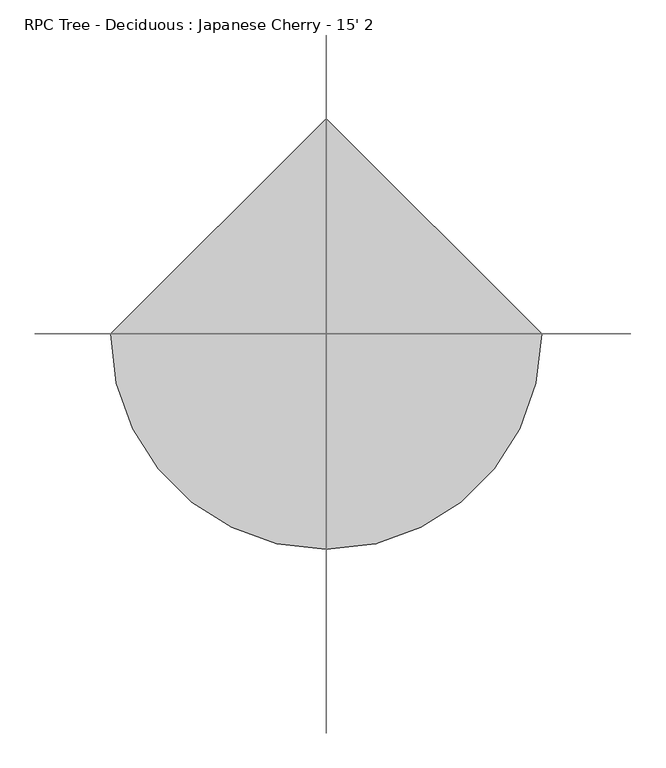
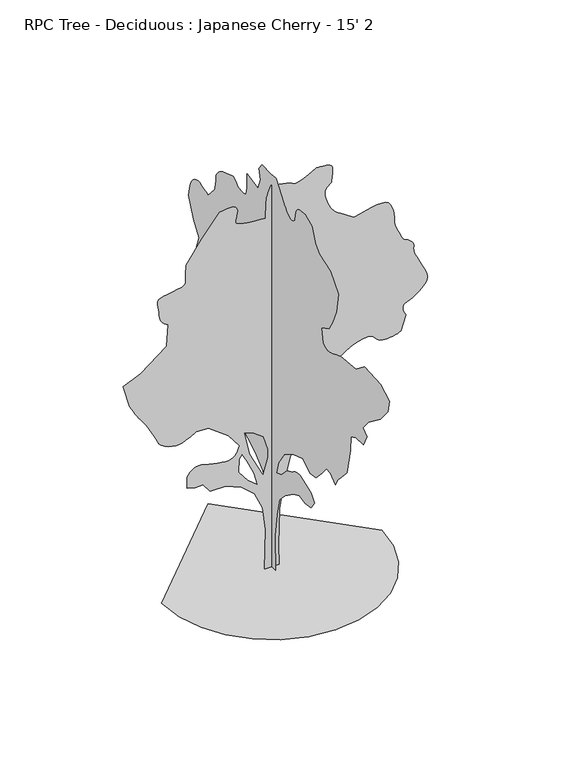
"""IFC4 building model written with IfcOpenShell, lengths in millimetres: geographic element geometry, RPC Tree - Deciduous : Japanese Cherry - 15' 2."""

from ifc_helpers import new_model, si_unit, origin, place, context, project, spatial, triangles, source, transform, mapped, element, save


def rpc_tree_deciduous_japanese_cherry_15_2_e499737d(model_context):
    return source(origin(), model_context, "Body", "Tessellation", [
        triangles([(-0.0028028, 75.7657196, 0.0059537), (-0.0028028, -73.2478183, 0.0059537), (-0.0028028, -59.7012251, 399.6312029), (-0.0028028, -100.3410047, 663.7914597), (-0.0028028, -147.7544623, 866.9916292), (-0.0028028, -256.1287339, 982.1375078), (-0.0028028, -418.6863261, 1097.2859299), (-0.0028028, -527.0605977, 1144.6976435), (-0.0028028, -635.434833, 1124.3775902), (-0.0028028, -750.5807842, 1144.6976435), (-0.0028028, -811.5407988, 1232.7519344), (-0.0028028, -750.5807842, 1314.0320023), (-0.0028028, -533.8347845, 1388.5377743), (-0.0028028, -514.9955638, 1387.0189716), (-0.0028028, -496.3341665, 1385.0834793), (-0.0028028, -478.0283798, 1382.3173691), (-0.0028028, -460.2559908, 1378.3091835), (-0.0028028, -443.1947865, 1372.6425236), (-0.0028028, -427.0200471, 1364.9005543), (-0.0028028, -411.9146828, 1354.6719635), (-0.0028028, -396.8067387, 1343.65345), (-0.0028028, -380.6345427, 1333.6991158), (-0.0028028, -363.5733384, 1324.6364422), (-0.0028028, -345.8009494, 1316.2824463), (-0.0028028, -327.4951627, 1308.4643188), (-0.0028028, -308.8337654, 1300.9992222), (-0.0028028, -289.994581, 1293.7118763), (-0.0028028, -188.3942419, 1185.3376774), (-0.0028028, -86.7944115, 1144.6976435), (-0.0028028, -127.4344454, 1286.9377258), (-0.0028028, -242.580869, 1456.2720119), (-0.0028028, -405.140496, 1557.8722057), (-0.0028028, -594.794799, 1618.8321476), (-0.0028028, -730.2607309, 1530.7779293), (-0.0028028, -838.6350025, 1544.3263756), (-0.0028028, -953.7809538, 1666.2439339), (-0.0028028, -1041.8351721, 1774.6181328), (-0.0028028, -1123.1126965, 1767.8439823), (-0.0028028, -1211.1669147, 1686.5663853), (-0.0028028, -1265.3528515, 1781.3922832), (-0.0028028, -1326.3127934, 1849.1240501), (-0.0028028, -1434.6871376, 1964.2723995), (-0.0028028, -1502.4187592, 2269.0726902), (-0.0028028, -1509.193055, 2431.6328259), (-0.0028028, -1604.0214237, 2472.2703163), (-0.0028028, -1753.0332584, 2485.8186172), (-0.0028028, -1813.9932003, 2614.5002975), (-0.0028028, -1739.4874283, 2675.4602394), (-0.0028028, -1841.0874767, 2797.3804138), (-0.0028028, -2071.3792339, 2973.5042564), (-0.0028028, -2220.3935394, 3149.6025192), (-0.0028028, -2247.4851997, 3291.8426743), (-0.0028028, -2078.1535297, 3386.6610146), (-0.0028028, -1766.5790886, 3400.2244308), (-0.0028028, -1610.7931034, 3278.3045471), (-0.0028028, -1312.7669632, 3244.4208595), (-0.0028028, -1272.2845505, 3228.5456657), (-0.0028028, -1232.7519344, 3213.2041603), (-0.0028028, -1195.1115721, 3198.9294502), (-0.0028028, -1160.3186377, 3186.2546425), (-0.0028028, -1129.3153702, 3175.7137161), (-0.0028028, -1103.0517843, 3167.8397781), (-0.0028028, -1082.4726625, 3163.1406464), (-0.0028028, -1064.0500225, 3162.8865921), (-0.0028028, -1044.5580437, 3166.9000099), (-0.0028028, -1025.4242552, 3173.6309944), (-0.0028028, -1008.065867, 3181.5558014), (-0.0028028, -993.907865, 3189.1248161), (-0.0028028, -984.3701477, 3194.789296), (-0.0028028, -980.8726141, 3197.024334), (-0.0028028, -947.0067307, 3359.5844696), (-0.0028028, -1089.2468857, 3434.0828293), (-0.0028028, -1156.9810507, 3542.4645859), (-0.0028028, -1231.4868954, 3718.5628487), (-0.0028028, -1272.127002, 3942.0832169), (-0.0028028, -1116.3410168, 4118.1814796), (-0.0028028, -913.1409199, 4192.7051285), (-0.0028028, -831.8608521, 4267.2034882), (-0.0028028, -770.9007648, 4429.7636238), (-0.0028028, -628.6606825, 4483.9417122), (-0.0028028, -605.4958537, 4483.8402649), (-0.0028028, -582.6891789, 4483.1542603), (-0.0028028, -560.5911455, 4481.2747238), (-0.0028028, -539.5599438, 4477.6426781), (-0.0028028, -519.9511116, 4471.5974075), (-0.0028028, -502.1202959, 4462.6310944), (-0.0028028, -486.4205638, 4450.0836044), (-0.0028028, -473.6824242, 4434.3863068), (-0.0028028, -464.1447433, 4416.5554184), (-0.0028028, -457.2740144, 4396.9467316), (-0.0028028, -452.5343691, 4375.9154572), (-0.0028028, -449.3949532, 4353.8173874), (-0.0028028, -447.3197528, 4331.0083145), (-0.0028028, -445.7805299, 4307.8434494), (-0.0028028, -434.0914178, 4294.9401672), (-0.0028028, -421.9248276, 4283.0531021), (-0.0028028, -408.8133096, 4273.1978897), (-0.0028028, -394.279422, 4266.3398781), (-0.0028028, -377.850701, 4263.5202827), (-0.0028028, -359.0495956, 4265.7303223), (-0.0028028, -337.4062583, 4273.9853416), (-0.0028028, -315.9610193, 4285.9741447), (-0.0028028, -297.7161846, 4298.6995308), (-0.0028028, -282.1358129, 4312.0091835), (-0.0028028, -268.6864885, 4325.8013649), (-0.0028028, -256.8373934, 4339.9237587), (-0.0028028, -246.0563473, 4354.3002068), (-0.0028028, -235.8074452, 4368.8033913), (-0.0028028, -140.9810386, 4497.5054192), (-0.0028028, -80.0209877, 4572.0037788), (-0.0028028, 21.579147, 4565.2219254), (-0.0028028, 184.1389784, 4572.0037788), (-0.0028028, 245.0987749, 4490.7235657), (-0.0028028, 218.0055885, 4375.5852448), (-0.0028028, 265.4200454, 4246.8835075), (-0.0028028, 475.3918765, 4287.5234688), (-0.0028028, 475.3918765, 4138.5014603), (-0.0028028, 476.9514107, 4115.4383331), (-0.0028028, 479.1637756, 4093.1623672), (-0.0028028, 482.6791134, 4072.5630432), (-0.0028028, 488.1502911, 4054.4781006), (-0.0028028, 496.2249435, 4039.6699928), (-0.0028028, 507.5609885, 4029.0273285), (-0.0028028, 522.8060609, 4023.3631393), (-0.0028028, 540.2228757, 4021.2551285), (-0.0028028, 557.6396542, 4020.5691238), (-0.0028028, 575.056469, 4021.0519432), (-0.0028028, 592.4732474, 4022.4995293), (-0.0028028, 609.8900259, 4024.6586998), (-0.0028028, 627.3093842, 4027.2748192), (-0.0028028, 644.726199, 4030.1449928), (-0.0028028, 660.7002239, 4045.9437378), (-0.0028028, 676.7352917, 4060.8791634), (-0.0028028, 692.8896835, 4074.0362091), (-0.0028028, 709.2193554, 4084.5265572), (-0.0028028, 725.7878208, 4091.4607269), (-0.0028028, 742.6534338, 4093.9498192), (-0.0028028, 759.8720776, 4091.1049347), (-0.0028028, 942.7522665, 4030.1449928), (-0.0028028, 968.7009007, 4012.6698967), (-0.0028028, 993.5827394, 3994.8390083), (-0.0028028, 1016.3309875, 3976.2971169), (-0.0028028, 1035.8813931, 3956.6881393), (-0.0028028, 1051.1646172, 3935.6568649), (-0.0028028, 1061.1163353, 3912.8477921), (-0.0028028, 1064.6722956, 3887.9048378), (-0.0028028, 1065.462291, 3862.3526184), (-0.0028028, 1067.6745832, 3837.8921928), (-0.0028028, 1071.0705969, 3814.3209572), (-0.0028028, 1075.4140091, 3791.4610153), (-0.0028028, 1080.4685698, 3769.1088913), (-0.0028028, 1085.9981741, 3747.1381393), (-0.0028028, 1091.7640285, 3725.3447021), (-0.0028028, 1220.4582081, 3583.1045471), (-0.0028028, 1259.5970982, 3600.2497215), (-0.0028028, 1298.4413841, 3615.8705704), (-0.0028028, 1336.691375, 3628.418351), (-0.0028028, 1374.0521759, 3636.343158), (-0.0028028, 1410.2294735, 3638.0956673), (-0.0028028, 1444.9259022, 3632.1521347), (-0.0028028, 1477.8442417, 3616.9629456), (-0.0028028, 1506.4193871, 3593.4931572), (-0.0028028, 1528.9517326, 3564.3086014), (-0.0028028, 1546.4471764, 3530.3996246), (-0.0028028, 1559.9143776, 3492.7059952), (-0.0028028, 1570.361269, 3452.1674812), (-0.0028028, 1578.7941845, 3409.7241417), (-0.0028028, 1586.218586, 3366.3410339), (-0.0028028, 1498.1643677, 3136.0643921), (-0.0028028, 1389.7926395, 2987.0423836), (-0.0028028, 1477.8442417, 2743.2023254), (-0.0028028, 1396.5641739, 2614.5002975), (-0.0028028, 1363.3893093, 2602.8164177), (-0.0028028, 1331.4588455, 2590.6497185), (-0.0028028, 1302.0151485, 2577.543251), (-0.0028028, 1276.3027645, 2563.0144867), (-0.0028028, 1255.5687103, 2546.5806061), (-0.0028028, 1241.0552067, 2527.7820442), (-0.0028028, 1234.0040382, 2506.1385979), (-0.0028028, 1231.6953129, 2483.1135498), (-0.0028028, 1230.4506214, 2460.4416779), (-0.0028028, 1230.0949745, 2438.0692062), (-0.0028028, 1230.4506214, 2415.9330574), (-0.0028028, 1231.339666, 2393.9721886), (-0.0028028, 1232.5842121, 2372.13326), (-0.0028028, 1234.0040382, 2350.3502872), (-0.0028028, 1206.9124506, 2241.9785591), (-0.0028028, 1017.2581112, 2262.2985397), (-0.0028028, 1001.4999161, 2230.5052769), (-0.0028028, 986.9863398, 2199.5401611), (-0.0028028, 974.9594576, 2170.2361359), (-0.0028028, 966.6663591, 2143.4188774), (-0.0028028, 963.3491198, 2119.9211838), (-0.0028028, 966.2523582, 2100.5664059), (-0.0028028, 976.6180773, 2086.1925739), (-0.0028028, 993.4227201, 2074.2646683), (-0.0028028, 1014.0196461, 2062.1005852), (-0.0028028, 1037.2225176, 2050.292149), (-0.0028028, 1061.8478313, 2039.431184), (-0.0028028, 1086.7093952, 2030.1093693), (-0.0028028, 1110.6234879, 2022.9211452), (-0.0028028, 1132.4039898, 2018.4583363), (-0.0028028, 1152.1322187, 2014.567004), (-0.0028028, 1170.7936523, 2008.9003441), (-0.0028028, 1188.5660414, 2001.7526699), (-0.0028028, 1205.6272093, 1993.4190216), (-0.0028028, 1222.157523, 1984.1961834), (-0.0028028, 1238.3297916, 1974.3816662), (-0.0028028, 1254.3241642, 1964.2723995), (-0.0028028, 1410.1126202, 2045.5524673), (-0.0028028, 1454.8979679, 2056.9850544), (-0.0028028, 1498.4412403, 2067.3533169), (-0.0028028, 1539.4952751, 2075.5879887), (-0.0028028, 1576.817997, 2080.6222744), (-0.0028028, 1609.1650051, 2081.3919949), (-0.0028028, 1635.2914627, 2076.8326801), (-0.0028028, 1653.9502075, 2065.8725933), (-0.0028028, 1666.2946575, 2049.9747265), (-0.0028028, 1674.7249569, 2031.5900928), (-0.0028028, 1679.8989143, 2011.1329113), (-0.0028028, 1682.4669262, 1989.0146393), (-0.0028028, 1683.0789528, 1965.6542919), (-0.0028028, 1682.3881519, 1941.4631813), (-0.0028028, 1681.0444839, 1916.8582878), (-0.0028028, 1657.7627655, 1892.3904499), (-0.0028028, 1634.1255455, 1869.1697742), (-0.0028028, 1609.7770317, 1848.4331039), (-0.0028028, 1584.3618679, 1831.4303627), (-0.0028028, 1557.5241165, 1819.4059513), (-0.0028028, 1528.9110374, 1813.5996197), (-0.0028028, 1498.1643677, 1815.2582394), (-0.0028028, 1465.6015297, 1822.4057682), (-0.0028028, 1432.5637207, 1830.9782101), (-0.0028028, 1400.2370602, 1839.0732101), (-0.0028028, 1369.8078129, 1844.8009129), (-0.0028028, 1342.4571568, 1846.2614342), (-0.0028028, 1319.3735367, 1841.5624477), (-0.0028028, 1301.7382759, 1828.8040695), (-0.0028028, 1288.4084209, 1812.3752758), (-0.0028028, 1277.2120113, 1797.7219551), (-0.0028028, 1267.7912201, 1784.5521194), (-0.0028028, 1259.7953419, 1772.5657871), (-0.0028028, 1252.8636429, 1761.4660286), (-0.0028028, 1246.6430923, 1750.9605652), (-0.0028028, 1240.778334, 1740.752322), (-0.0028028, 1263.8618088, 1737.6916077), (-0.0028028, 1286.1172817, 1733.6834221), (-0.0028028, 1306.714135, 1727.7779686), (-0.0028028, 1324.821896, 1719.0302467), (-0.0028028, 1339.6122723, 1706.4901691), (-0.0028028, 1350.2574074, 1689.2105553), (-0.0028028, 1355.9242126, 1666.2439339), (-0.0028028, 1358.2355541, 1639.3300243), (-0.0028028, 1359.4802456, 1610.9912018), (-0.0028028, 1359.8357471, 1581.4687305), (-0.0028028, 1359.4802456, 1550.9989334), (-0.0028028, 1358.591201, 1519.8178425), (-0.0028028, 1357.3466549, 1488.1643967), (-0.0028028, 1355.9242126, 1456.2720119), (-0.0028028, 1321.1312782, 1430.3436527), (-0.0028028, 1286.5720505, 1405.5990875), (-0.0028028, 1252.4876484, 1383.2266159), (-0.0028028, 1219.1146128, 1364.4078518), (-0.0028028, 1186.6915192, 1350.328624), (-0.0028028, 1155.4494581, 1342.1725811), (-0.0028028, 1125.6323828, 1341.1261333), (-0.0028028, 1095.812764, 1344.8167511), (-0.0028028, 1064.5732464, 1349.9322819), (-0.0028028, 1032.1476093, 1356.2316067), (-0.0028028, 998.774501, 1363.478112), (-0.0028028, 964.6902443, 1371.4385273), (-0.0028028, 930.1334873, 1379.8688267), (-0.0028028, 895.3380095, 1388.5377743), (-0.0028028, 692.1378399, 1341.1261333), (-0.0028028, 455.0718596, 1219.2061043), (-0.0028028, 319.6059277, 1144.6976435), (-0.0028028, 163.8189614, 1016.005862), (-0.0028028, 68.9922959, 819.5799156), (-0.0028028, 41.8991095, 541.8713216), (-0.0028028, 68.9922959, 264.1652892), (80.2102203, 0.0002552, 0.0), (-82.349661, 0.0002552, 0.0), (-68.8030678, 0.0002233, 460.5862032), (-102.6694236, 0.000202, 724.7463873), (-190.7229152, 0.0001914, 914.3981833), (-332.9637969, 0.0001914, 1043.0925081), (-509.0697627, 0.0001807, 1117.5983528), (-678.4015417, 0.0001807, 1117.5983528), (-759.684153, 0.0001807, 1219.1984013), (-847.7358278, 0.0001807, 1219.1984013), (-935.7901188, 0.0001807, 1239.5183819), (-935.7901188, 0.0001701, 1368.2127068), (-918.2539072, 0.0001701, 1391.2175526), (-900.0065472, 0.0001701, 1412.9192802), (-880.3392883, 0.0001595, 1432.0150623), (-858.5384388, 0.0001595, 1447.2017807), (-833.8928501, 0.0001595, 1457.1737011), (-805.6936993, 0.0001595, 1460.6307575), (-773.2299831, 0.0001595, 1456.266925), (-734.6829174, 0.0001595, 1446.5108345), (-690.4487715, 0.0001595, 1435.4516258), (-643.1335636, 0.0001701, 1424.2757092), (-595.3460009, 0.0001701, 1414.1639717), (-549.689449, 0.0001701, 1406.3051491), (-508.7725788, 0.0001701, 1401.8804192), (-475.2013721, 0.0001701, 1402.0785175), (-448.544024, 0.0001701, 1408.1415195), (-426.1513865, 0.0001701, 1419.8916744), (-407.3122021, 0.0001595, 1436.3813656), (-391.3152497, 0.0001595, 1456.660651), (-377.4544679, 0.0001595, 1479.7848209), (-365.0135485, 0.0001595, 1504.8039333), (-353.2838139, 0.0001595, 1530.7728424), (-475.2013721, 0.0001488, 1693.3329781), (-698.7215223, 0.0001382, 1855.8931137), (-834.1899977, 0.0001382, 1862.6647934), (-856.0492739, 0.0001382, 1849.6320133), (-878.4419477, 0.0001382, 1836.7771294), (-901.9038877, 0.0001382, 1824.277747), (-926.9610065, 0.0001382, 1812.3092915), (-954.1543322, 0.0001382, 1801.0544552), (-984.01203, 0.0001382, 1790.6861927), (-1017.0701866, 0.0001488, 1781.3847256), (-1055.1015862, 0.0001488, 1778.1664627), (-1097.4002398, 0.0001488, 1784.6638859), (-1140.7656887, 0.0001382, 1798.9792912), (-1182.0000904, 0.0001382, 1819.2206429), (-1217.9005154, 0.0001382, 1843.490237), (-1245.2690483, 0.0001382, 1869.8935673), (-1260.907774, 0.0001382, 1896.5332203), (-1274.5551968, 0.0001382, 1929.7461639), (-1296.2570698, 0.0001276, 1973.9803825), (-1323.2903034, 0.0001276, 2024.4959038), (-1352.9320988, 0.0001276, 2076.5482498), (-1382.45457, 0.0001276, 2125.4025352), (-1409.1321568, 0.0001169, 2166.3195145), (-1430.2420601, 0.0001169, 2194.5592152), (-1448.055217, 0.0001169, 2217.0508656), (-1466.5769062, 0.0001169, 2243.4541958), (-1485.6928905, 0.0001169, 2273.113868), (-1505.2813751, 0.0001169, 2305.3794857), (-1525.2255066, 0.0001063, 2339.6035595), (-1545.4082863, 0.0001063, 2375.12799), (-1565.7080647, 0.0001063, 2411.3051422), (-1640.2164528, 9.57e-05, 2668.7039658), (-1443.7878902, 8.51e-05, 2749.9838882), (-1159.310269, 7.44e-05, 2973.5042564), (-1145.7618954, 5.32e-05, 3217.3190254), (-1165.9447477, 5.32e-05, 3231.9748169), (-1185.2970549, 5.32e-05, 3247.3163223), (-1202.9906696, 5.32e-05, 3264.0804153), (-1218.1951195, 5.32e-05, 3282.9780991), (-1230.0823299, 5.32e-05, 3304.7203766), (-1237.8242992, 5.32e-05, 3330.0188324), (-1240.5902641, 5.32e-05, 3359.5591805), (-1243.0389519, 4.25e-05, 3392.8330215), (-1248.5659401, 4.25e-05, 3427.5294502), (-1254.4511913, 4.25e-05, 3461.7686394), (-1257.9665291, 4.25e-05, 3493.6204742), (-1256.3865383, 4.25e-05, 3521.204837), (-1246.9860947, 4.25e-05, 3542.6169022), (-1227.0419632, 4.25e-05, 3556.002713), (-1192.1092844, 4.25e-05, 3564.4103394), (-1144.1438982, 3.19e-05, 3572.715937), (-1090.0164608, 3.19e-05, 3581.5808029), (-1036.6002445, 3.19e-05, 3591.7915169), (-990.7659056, 3.19e-05, 3603.9835052), (-959.3867163, 3.19e-05, 3618.9186401), (-949.3359489, 3.19e-05, 3637.2829262), (-951.449192, 3.19e-05, 3659.3809959), (-952.1400656, 3.19e-05, 3684.6794518), (-951.644747, 3.19e-05, 3712.6448959), (-950.2045732, 3.19e-05, 3742.718351), (-948.0532511, 2.13e-05, 3774.4175789), (-945.4268852, 2.13e-05, 3807.1836021), (-942.5617258, 2.13e-05, 3840.4830231), (-773.2299831, 1.06e-05, 4084.3233719), (-576.803964, -1.06e-05, 4328.16343), (-534.9980856, -1.06e-05, 4335.1231796), (-494.9117606, -1.06e-05, 4340.3809982), (-458.2595647, -1.06e-05, 4342.2096657), (-426.7635221, -1.06e-05, 4338.8569633), (-402.1382083, -1.06e-05, 4328.6459587), (-386.1031769, -1.06e-05, 4309.850013), (-380.3754742, 0.0, 4280.7416153), (-383.1999384, 0.0, 4247.9503029), (-389.6972889, 0.0, 4219.0450905), (-396.9057878, 0.0, 4193.848082), (-401.8613357, 0.0, 4172.0549355), (-401.6048106, 0.0, 4153.462175), (-393.1720041, 0.0, 4137.8410355), (-373.6038308, 0.0, 4124.9633331), (-343.9238837, 0.0, 4114.5238541), (-307.8431645, 0.0, 4106.2435455), (-266.4335192, 1.06e-05, 4099.7157463), (-220.7586908, 1.06e-05, 4094.6355331), (-171.883967, 1.06e-05, 4090.5971169), (-120.8766607, 1.06e-05, 4087.2697037), (-68.8030678, 1.06e-05, 4084.3233719), (-62.0293897, 0.0, 4267.2034882), (-60.4495079, -1.06e-05, 4293.1367889), (-56.0260951, -1.06e-05, 4318.689299), (-49.2331141, -1.06e-05, 4343.962175), (-40.544273, -1.06e-05, 4369.0065765), (-30.4335416, -1.06e-05, 4393.8733727), (-19.3751868, -1.06e-05, 4418.612851), (-7.8427643, -1.06e-05, 4443.3017509), (38.3857792, -1.06e-05, 4434.5642029), (83.3110485, -1.06e-05, 4425.7249168), (125.6295138, -1.06e-05, 4416.6571564), (164.0381523, -1.06e-05, 4407.2083145), (197.2334371, -1.06e-05, 4397.3022331), (223.9120957, -1.06e-05, 4386.7865959), (242.7705922, -1.06e-05, 4375.5599556), (267.3174405, -1.06e-05, 4372.2834114), (307.2640574, -1.06e-05, 4382.5194145), (355.6256767, -1.06e-05, 4401.5188362), (405.4097383, -1.06e-05, 4424.5566742), (449.6235366, -1.06e-05, 4446.8576385), (481.2770551, -2.13e-05, 4463.7234695), (493.3827115, -2.13e-05, 4470.4035851), (503.1388384, -2.13e-05, 4470.6067703), (528.2975498, -2.13e-05, 4470.3274269), (562.6967946, -2.13e-05, 4468.2699944), (600.177065, -2.13e-05, 4463.1392029), (634.5763098, -1.06e-05, 4453.6142029), (659.7350212, -1.06e-05, 4438.3994339), (669.4911844, -1.06e-05, 4416.1999168), (669.0949877, -1.06e-05, 4390.4698013), (667.9900406, -1.06e-05, 4365.4506889), (666.2907984, -1.06e-05, 4341.0411324), (664.1190559, -1.06e-05, 4317.089106), (661.5918119, -1.06e-05, 4293.4922905), (658.8257017, 0.0, 4270.1245308), (655.9428108, 0.0, 4246.8835075), (638.6835445, 0.0, 4233.6753021), (622.3741476, 0.0, 4219.7308044), (607.9571134, 0.0, 4204.2114029), (596.3848546, 0.0, 4186.4060944), (588.6048426, 0.0, 4165.5271362), (585.5644395, 0.0, 4140.7876579), (588.2111166, 0.0, 4111.3996262), (595.5949319, 1.06e-05, 4078.8367882), (605.8235227, 1.06e-05, 4045.6643944), (618.4244614, 1.06e-05, 4012.9492401), (632.9176901, 1.06e-05, 3981.7834099), (648.8333611, 1.06e-05, 3953.233699), (665.698974, 1.06e-05, 3928.3416138), (683.0370146, 2.13e-05, 3908.1995293), (703.4154945, 2.13e-05, 3889.8099541), (729.1278786, 2.13e-05, 3869.6170006), (759.2802532, 2.13e-05, 3847.9505905), (792.9912043, 2.13e-05, 3825.1159378), (829.3639841, 2.13e-05, 3801.3670967), (867.5148531, 2.13e-05, 3777.0592781), (906.5572374, 2.13e-05, 3752.4212471), (974.48703, 2.13e-05, 3771.0140076), (1040.6997763, 2.13e-05, 3787.8795479), (1103.475959, 2.13e-05, 3801.2909386), (1161.1010027, 2.13e-05, 3809.5712471), (1211.8502306, 2.13e-05, 3810.9682549), (1254.0116833, 2.13e-05, 3803.7800308), (1285.8633728, 2.13e-05, 3786.2793549), (1308.8096466, 2.13e-05, 3757.831382), (1325.9495888, 3.19e-05, 3721.2045479), (1338.1136719, 3.19e-05, 3679.8280037), (1346.1325138, 3.19e-05, 3637.155899), (1350.8315002, 3.19e-05, 3596.6173851), (1353.0438652, 4.25e-05, 3561.641613), (1353.5976105, 4.25e-05, 3535.6827324), (1358.8503422, 4.25e-05, 3507.9969223), (1372.3961723, 4.25e-05, 3469.2870758), (1390.9178616, 4.25e-05, 3425.1418053), (1411.1006413, 5.32e-05, 3381.0982727), (1429.6249466, 5.32e-05, 3342.7442184), (1443.1707767, 5.32e-05, 3315.6423843), (1448.4235085, 5.32e-05, 3305.3808014), (1455.5126106, 5.32e-05, 3302.5614967), (1473.6202263, 5.32e-05, 3294.4079247), (1498.0094353, 5.32e-05, 3281.4031952), (1523.9376492, 5.32e-05, 3264.0042572), (1546.6656223, 5.32e-05, 3242.6936394), (1561.456144, 5.32e-05, 3217.9538704), (1563.5693871, 6.38e-05, 3190.2424805), (1560.9227463, 6.38e-05, 3161.8962456), (1563.9655838, 6.38e-05, 3134.3880409), (1571.7456322, 6.38e-05, 3106.8795456), (1583.3178909, 6.38e-05, 3078.5585999), (1597.7324181, 6.38e-05, 3048.5613029), (1614.0443584, 7.44e-05, 3016.0746231), (1631.3036247, 7.44e-05, 2980.2605301), (1651.0114334, 7.44e-05, 2941.4239471), (1672.8529781, 7.44e-05, 2900.911013), (1693.1526112, 7.44e-05, 2859.5850471), (1708.2377369, 8.51e-05, 2818.2593719), (1714.4404106, 8.51e-05, 2777.7461472), (1708.0801884, 8.51e-05, 2738.9095642), (1685.4894161, 8.51e-05, 2702.5620735), (1655.0603142, 9.57e-05, 2670.8884254), (1626.9983643, 9.57e-05, 2644.9042557), (1600.3587112, 9.57e-05, 2623.6442162), (1574.1941746, 9.57e-05, 2606.1944092), (1547.5546669, 9.57e-05, 2591.5894867), (1519.4951878, 9.57e-05, 2578.8641006), (1489.0634697, 9.57e-05, 2567.103772), (1463.2545799, 9.57e-05, 2553.5147758), (1448.4615875, 9.57e-05, 2536.3646599), (1442.8532089, 9.57e-05, 2516.2632706), (1444.5930737, 0.0001063, 2493.7893517), (1451.8397243, 0.0001063, 2469.5399597), (1462.7592613, 0.0001063, 2444.1069191), (1475.5176395, 0.0001063, 2418.079438), (1421.329232, 0.0001169, 2248.7450066), (1402.2741451, 0.0001169, 2240.1167542), (1382.0913654, 0.0001169, 2231.9607113), (1359.6579964, 0.0001169, 2224.752285), (1333.8491066, 0.0001169, 2218.9661556), (1303.5367126, 0.0001169, 2215.0772942), (1267.5955925, 0.0001169, 2213.5558754), (1224.9032856, 0.0001169, 2214.8791958), (1186.5543182, 0.0001169, 2223.6651421), (1160.2907324, 0.0001169, 2241.2216286), (1139.9504042, 0.0001169, 2263.0426804), (1119.3738258, 0.0001169, 2284.6250839), (1092.3990189, 0.0001169, 2301.470422), (1052.8638594, 0.0001169, 2309.0727196), (994.6089123, 0.0001169, 2302.9309433), (927.2531399, 0.0001169, 2283.7970821), (865.4625074, 0.0001169, 2256.8426228), (810.6645441, 0.0001169, 2224.1985397), (764.2764599, 0.0001169, 2188.0035107), (727.7258566, 0.0001169, 2150.3835686), (702.4274008, 0.0001276, 2113.4772457), (689.8112377, 0.0001276, 2079.4133366), (689.5343651, 0.0001276, 2049.0602474), (699.2092106, 0.0001276, 2021.5520428), (717.179698, 0.0001276, 1996.4136063), (741.7847368, 0.0001276, 1973.172583), (771.3655621, 0.0001382, 1951.3515312), (804.2662428, 0.0001382, 1930.4778053), (838.8229998, 0.0001382, 1910.0790504), (858.9855045, 0.0001382, 1896.9268009), (878.2006107, 0.0001382, 1883.2412991), (895.5183764, 0.0001382, 1868.4914726), (909.9938009, 0.0001382, 1852.1415985), (920.6770878, 0.0001382, 1833.6579884), (926.620693, 0.0001382, 1812.5073898), (926.8772181, 0.0001382, 1788.158876), (924.1721506, 0.0001488, 1758.4790016), (921.8225847, 0.0001488, 1722.4008259), (919.7677683, 0.0001488, 1680.9911442), (917.9516727, 0.0001488, 1635.3142811), (916.3107845, 0.0001595, 1586.4395027), (914.7919092, 0.0001595, 1535.4337498), (913.3288445, 0.0001595, 1483.3585854), (878.4571358, 0.0001595, 1457.529348), (843.3467062, 0.0001595, 1433.4780544), (807.7613056, 0.0001701, 1412.980323), (771.4646839, 0.0001701, 1397.8139523), (734.2231344, 0.0001701, 1389.7570312), (695.792922, 0.0001701, 1390.585033), (655.9428108, 0.0001701, 1402.0785175), (615.8971447, 0.0001701, 1417.3236626), (576.9157305, 0.0001701, 1428.6597439), (538.820781, 0.0001595, 1436.7368671), (501.4395962, 0.0001595, 1442.205574), (464.5917727, 0.0001595, 1445.7209118), (428.0995597, 0.0001595, 1447.9332767), (391.7826267, 0.0001595, 1449.4927746), (276.6366936, 0.0001701, 1374.9868572), (202.1305764, 0.0001807, 1205.6525711), (127.6236689, 0.0001914, 921.1724064), (86.9838894, 0.0002126, 643.4663195), (73.4370464, 0.0002339, 237.0665254), (-95.8962542, 8.51e-05, 1097.2783722), (-41.7096271, 7.44e-05, 1286.9326389), (-41.7096271, 6.38e-05, 1381.7585369), (-89.122576, 5.32e-05, 1544.3186726), (-211.0424234, 5.32e-05, 1632.3728909), (-305.8695931, 5.32e-05, 1666.238847), (-244.9095423, 6.38e-05, 1395.3069832), (-156.8557963, 6.38e-05, 1009.2266247), (-197.4958302, 6.38e-05, 1158.2383867), (-272.003746, 5.32e-05, 1320.7984497), (-326.1896101, 4.25e-05, 1422.3986435), (-360.0554572, 4.25e-05, 1374.9868572), (-366.829644, 5.32e-05, 1225.9725517), (-265.2295592, 6.38e-05, 1097.2783722), (-1212.9170259, 0.0, 0.0045929), (-1180.85205, -277.9194097, 0.0045929), (-1089.5287725, -533.1464181, 0.0045929), (-946.2625174, -758.3633034, 0.0045929), (-758.3633034, -946.2625174, 0.0045929), (-533.1464181, -1089.5287725, 0.0045929), (-277.9194097, -1180.85205, 0.0045929), (5.3e-05, -1212.9170259, 0.0045929), (277.9194097, -1180.85205, 0.0045929), (533.1464181, -1089.5287725, 0.0045929), (758.3633034, -946.2625174, 0.0045929), (946.2625174, -758.3633034, 0.0045929), (1089.5287725, -533.1464181, 0.0045929), (1180.85205, -277.9194097, 0.0045929), (1212.9170259, 0.0001063, 0.0045929), (-0.0001591, 1212.9170259, 0.0045929)], [[38, 39, 40], [115, 116, 117], [1, 2, 3], [280, 1, 3], [279, 280, 3], [279, 3, 4], [278, 279, 4], [278, 4, 5], [186, 187, 188], [277, 278, 5], [46, 47, 48], [45, 46, 48], [277, 5, 6], [185, 186, 188], [10, 11, 12], [9, 10, 12], [9, 12, 13], [8, 9, 13], [8, 13, 14], [8, 14, 15], [8, 15, 16], [8, 16, 17], [8, 17, 18], [8, 18, 19], [8, 19, 20], [8, 20, 21], [7, 8, 21], [7, 21, 22], [7, 22, 23], [7, 23, 24], [7, 24, 25], [7, 25, 26], [6, 7, 26], [6, 26, 27], [6, 27, 28], [277, 6, 28], [277, 28, 29], [51, 52, 53], [50, 51, 53], [50, 53, 54], [50, 54, 55], [49, 50, 55], [49, 55, 56], [48, 49, 56], [48, 56, 57], [45, 48, 57], [44, 45, 57], [44, 57, 58], [44, 58, 59], [44, 59, 60], [44, 60, 61], [44, 61, 62], [44, 62, 63], [276, 277, 29], [276, 29, 30], [184, 185, 188], [183, 184, 188], [44, 63, 64], [115, 117, 118], [111, 112, 113], [111, 113, 114], [182, 183, 188], [109, 110, 111], [109, 111, 114], [108, 109, 114], [108, 114, 115], [107, 108, 115], [106, 107, 115], [105, 106, 115], [104, 105, 115], [115, 118, 119], [170, 171, 172], [170, 172, 173], [170, 173, 174], [170, 174, 175], [74, 75, 76], [74, 76, 77], [73, 74, 77], [72, 73, 77], [71, 72, 77], [258, 259, 260], [181, 182, 188], [78, 79, 80], [170, 175, 176], [103, 104, 115], [78, 80, 81], [44, 64, 65], [275, 276, 30], [275, 30, 31], [274, 275, 31], [78, 81, 82], [78, 82, 83], [78, 83, 84], [78, 84, 85], [78, 85, 86], [78, 86, 87], [78, 87, 88], [78, 88, 89], [78, 89, 90], [78, 90, 91], [78, 91, 92], [78, 92, 93], [78, 93, 94], [78, 94, 95], [78, 95, 96], [71, 77, 78], [71, 78, 96], [71, 96, 97], [71, 97, 98], [71, 98, 99], [71, 99, 100], [115, 119, 120], [180, 181, 188], [38, 40, 41], [223, 224, 225], [33, 34, 35], [33, 35, 36], [33, 36, 37], [102, 103, 115], [179, 180, 188], [44, 65, 66], [170, 176, 177], [71, 100, 101], [43, 44, 66], [42, 43, 66], [41, 42, 66], [38, 41, 66], [37, 38, 66], [33, 37, 66], [33, 66, 67], [33, 67, 68], [33, 68, 69], [33, 69, 70], [32, 33, 70], [31, 32, 70], [274, 31, 70], [273, 274, 70], [273, 70, 71], [273, 71, 101], [273, 101, 102], [273, 102, 115], [273, 115, 120], [273, 120, 121], [273, 121, 122], [273, 122, 123], [273, 123, 124], [273, 124, 125], [273, 125, 126], [273, 126, 127], [273, 127, 128], [273, 128, 129], [273, 129, 130], [273, 130, 131], [272, 273, 131], [271, 272, 131], [270, 271, 131], [269, 270, 131], [268, 269, 131], [268, 131, 132], [268, 132, 133], [268, 133, 134], [167, 168, 169], [257, 258, 260], [257, 260, 261], [256, 257, 261], [256, 261, 262], [255, 256, 262], [255, 262, 263], [254, 255, 263], [254, 263, 264], [254, 264, 265], [254, 265, 266], [254, 266, 267], [254, 267, 268], [253, 254, 268], [252, 253, 268], [251, 252, 268], [250, 251, 268], [249, 250, 268], [248, 249, 268], [247, 248, 268], [246, 247, 268], [245, 246, 268], [166, 167, 169], [165, 166, 169], [164, 165, 169], [163, 164, 169], [162, 163, 169], [161, 162, 169], [160, 161, 169], [159, 160, 169], [158, 159, 169], [157, 158, 169], [156, 157, 169], [155, 156, 169], [154, 155, 169], [154, 169, 170], [154, 170, 177], [153, 154, 177], [153, 177, 178], [153, 178, 179], [153, 179, 188], [222, 223, 225], [222, 225, 226], [221, 222, 226], [220, 221, 226], [219, 220, 226], [218, 219, 226], [217, 218, 226], [216, 217, 226], [215, 216, 226], [214, 215, 226], [213, 214, 226], [212, 213, 226], [212, 226, 227], [212, 227, 228], [212, 228, 229], [212, 229, 230], [212, 230, 231], [211, 212, 231], [211, 231, 232], [211, 232, 233], [210, 211, 233], [209, 210, 233], [209, 233, 234], [209, 234, 235], [209, 235, 236], [209, 236, 237], [209, 237, 238], [209, 238, 239], [209, 239, 240], [208, 209, 240], [208, 240, 241], [207, 208, 241], [206, 207, 241], [206, 241, 242], [205, 206, 242], [204, 205, 242], [204, 242, 243], [203, 204, 243], [202, 203, 243], [202, 243, 244], [201, 202, 244], [201, 244, 245], [201, 245, 268], [200, 201, 268], [199, 200, 268], [198, 199, 268], [197, 198, 268], [196, 197, 268], [195, 196, 268], [194, 195, 268], [153, 188, 189], [153, 189, 190], [152, 153, 190], [152, 190, 191], [151, 152, 191], [136, 137, 138], [135, 136, 138], [135, 138, 139], [134, 135, 139], [134, 139, 140], [134, 140, 141], [134, 141, 142], [134, 142, 143], [134, 143, 144], [134, 144, 145], [134, 145, 146], [134, 146, 147], [134, 147, 148], [134, 148, 149], [134, 149, 150], [134, 150, 151], [134, 151, 191], [134, 191, 192], [134, 192, 193], [268, 134, 193], [194, 268, 193], [583, 580, 581], [574, 281, 575], [580, 583, 584], [573, 574, 575], [583, 581, 575], [580, 584, 585], [572, 573, 575], [582, 583, 575], [582, 575, 281], [571, 572, 575], [571, 575, 576], [281, 282, 283], [570, 571, 576], [570, 576, 577], [344, 345, 346], [290, 291, 292], [406, 407, 408], [570, 577, 578], [290, 292, 293], [289, 290, 293], [289, 293, 294], [289, 294, 295], [289, 295, 296], [289, 296, 297], [289, 297, 298], [289, 298, 299], [289, 299, 300], [289, 300, 301], [289, 301, 302], [289, 302, 303], [288, 289, 303], [287, 288, 303], [287, 303, 304], [287, 304, 305], [287, 305, 306], [286, 287, 306], [286, 306, 307], [286, 307, 308], [286, 308, 309], [569, 570, 578], [554, 555, 556], [405, 406, 408], [343, 344, 346], [512, 513, 514], [511, 512, 514], [511, 514, 515], [511, 515, 516], [511, 516, 517], [510, 511, 517], [510, 517, 518], [510, 518, 519], [510, 519, 520], [510, 520, 521], [510, 521, 522], [510, 522, 523], [510, 523, 524], [509, 510, 524], [509, 524, 525], [508, 509, 525], [434, 435, 436], [342, 343, 346], [507, 508, 525], [507, 525, 526], [405, 408, 409], [404, 405, 409], [403, 404, 409], [403, 409, 410], [402, 403, 410], [401, 402, 410], [400, 401, 410], [400, 410, 411], [399, 400, 411], [399, 411, 412], [399, 412, 413], [399, 413, 414], [399, 414, 415], [377, 378, 379], [341, 342, 346], [341, 346, 347], [340, 341, 347], [339, 340, 347], [338, 339, 347], [337, 338, 347], [336, 337, 347], [335, 336, 347], [334, 335, 347], [333, 334, 347], [377, 379, 380], [377, 380, 381], [377, 381, 382], [377, 382, 383], [377, 383, 384], [377, 384, 385], [377, 385, 386], [377, 386, 387], [377, 387, 388], [377, 388, 389], [377, 389, 390], [377, 390, 391], [376, 377, 391], [376, 391, 392], [375, 376, 392], [374, 375, 392], [373, 374, 392], [372, 373, 392], [372, 392, 393], [371, 372, 393], [370, 371, 393], [369, 370, 393], [369, 393, 394], [369, 394, 395], [369, 395, 396], [332, 333, 347], [369, 396, 397], [426, 427, 428], [426, 428, 429], [425, 426, 429], [425, 429, 430], [424, 425, 430], [424, 430, 431], [423, 424, 431], [423, 431, 432], [422, 423, 432], [422, 432, 433], [421, 422, 433], [420, 421, 433], [419, 420, 433], [418, 419, 433], [418, 433, 434], [418, 434, 436], [418, 436, 437], [418, 437, 438], [418, 438, 439], [417, 418, 439], [417, 439, 440], [416, 417, 440], [416, 440, 441], [415, 416, 441], [399, 415, 441], [399, 441, 442], [399, 442, 443], [399, 443, 444], [399, 444, 445], [399, 445, 446], [399, 446, 447], [399, 447, 448], [399, 448, 449], [369, 397, 398], [331, 332, 347], [368, 369, 398], [360, 361, 362], [359, 360, 362], [359, 362, 363], [358, 359, 363], [358, 363, 364], [357, 358, 364], [357, 364, 365], [356, 357, 365], [355, 356, 365], [355, 365, 366], [354, 355, 366], [353, 354, 366], [352, 353, 366], [351, 352, 366], [350, 351, 366], [349, 350, 366], [348, 349, 366], [348, 366, 367], [348, 367, 368], [348, 368, 398], [347, 348, 398], [347, 398, 399], [347, 399, 449], [347, 449, 450], [347, 450, 451], [347, 451, 452], [331, 347, 452], [331, 452, 453], [331, 453, 454], [331, 454, 455], [331, 455, 456], [330, 331, 456], [329, 330, 456], [328, 329, 456], [327, 328, 456], [326, 327, 456], [325, 326, 456], [324, 325, 456], [323, 324, 456], [322, 323, 456], [321, 322, 456], [320, 321, 456], [319, 320, 456], [318, 319, 456], [317, 318, 456], [316, 317, 456], [315, 316, 456], [314, 315, 456], [314, 456, 457], [314, 457, 458], [314, 458, 459], [314, 459, 460], [314, 460, 461], [314, 461, 462], [314, 462, 463], [314, 463, 464], [314, 464, 465], [314, 465, 466], [314, 466, 467], [314, 467, 468], [314, 468, 469], [314, 469, 470], [314, 470, 471], [314, 471, 472], [314, 472, 473], [314, 473, 474], [314, 474, 475], [314, 475, 476], [314, 476, 477], [314, 477, 478], [314, 478, 479], [314, 479, 480], [314, 480, 481], [314, 481, 482], [314, 482, 483], [314, 483, 484], [314, 484, 485], [314, 485, 486], [314, 486, 487], [314, 487, 488], [314, 488, 489], [314, 489, 490], [314, 490, 491], [314, 491, 492], [314, 492, 493], [314, 493, 494], [314, 494, 495], [314, 495, 496], [314, 496, 497], [314, 497, 498], [314, 498, 499], [314, 499, 500], [314, 500, 501], [314, 501, 502], [580, 585, 586], [554, 556, 557], [553, 554, 557], [553, 557, 558], [553, 558, 559], [553, 559, 560], [553, 560, 561], [553, 561, 562], [553, 562, 563], [552, 553, 563], [552, 563, 564], [551, 552, 564], [550, 551, 564], [550, 564, 565], [549, 550, 565], [549, 565, 566], [548, 549, 566], [547, 548, 566], [546, 547, 566], [545, 546, 566], [544, 545, 566], [543, 544, 566], [542, 543, 566], [541, 542, 566], [540, 541, 566], [539, 540, 566], [538, 539, 566], [538, 566, 567], [537, 538, 567], [537, 567, 568], [537, 568, 569], [537, 569, 578], [536, 537, 578], [535, 536, 578], [535, 578, 579], [534, 535, 579], [534, 579, 580], [533, 534, 580], [532, 533, 580], [507, 526, 527], [506, 507, 527], [531, 532, 580], [506, 527, 528], [530, 531, 580], [281, 283, 284], [582, 281, 284], [582, 284, 285], [582, 285, 286], [588, 582, 286], [587, 588, 286], [587, 286, 309], [586, 587, 309], [586, 309, 310], [586, 310, 311], [586, 311, 312], [586, 312, 313], [580, 586, 313], [580, 313, 314], [530, 580, 314], [529, 530, 314], [502, 503, 504], [502, 504, 505], [314, 502, 505], [529, 314, 505], [529, 505, 506], [529, 506, 528], [603, 604, 589], [602, 603, 589], [602, 589, 590], [601, 602, 590], [601, 590, 591], [601, 591, 592], [600, 601, 592], [599, 600, 592], [599, 592, 593], [599, 593, 594], [599, 594, 595], [599, 595, 596], [599, 596, 597], [599, 597, 598]], closed=False),
    ])


if __name__ == "__main__":
    model = new_model("IFC4")
    model_context = context("Model", 3, world=origin())
    ifc_project = project(units=[si_unit("LENGTHUNIT", "METRE", prefix="MILLI")], contexts=[model_context])
    site = spatial("IfcSite", under=ifc_project)
    building = spatial("IfcBuilding", under=site)
    placement = place(None, origin())
    rpc_tree_deciduous_japanese_cherry_15_2_shape = rpc_tree_deciduous_japanese_cherry_15_2_e499737d(model_context)
    element("IfcGeographicElement", 1, ObjectType="RPC Tree - Deciduous : Japanese Cherry - 15' 2", at=placement, inside=building, context=model_context, shape_type="MappedRepresentation", body=[
        mapped(rpc_tree_deciduous_japanese_cherry_15_2_shape, transform((0.0, 0.0, 0.0), x_axis=(1.0, 0.0, 0.0), y_axis=(0.0, 1.0, 0.0), z_axis=(0.0, 0.0, 1.0))),
    ])
    save(model, "model.ifc")

# Revit data of these elements
# Type "RPC Tree - Deciduous : Japanese Cherry - 15' 2"
#   built-in parameter 1005198 = "{2, 15},{39, RPC-16-FXGW-2MQ0-PN7K-A000-ST1L-LVER-AU},{1, 0},{1, 0},{2, 35},{1, 8},{5, Color},{1, 0},{1, 0},{3, 0.8},{3, 0.8},{3, 0.8},{1, 8},{7, BBoxMin},{1, 0},{1, 0},{1, 0},{1, 0},{1, 0},{1, 8},{7, BBoxMax},{1, 0},{1, 0},{1, 0},{1, 0},{1, 0},{2, 11},{9, RPCTypeId},{1, 0},{1, 0},{39, RPC-16-FXGW-2MQ0-PN7K-A000-ST1L-LVER-AU},{1, 6},{14, RPCPlantHeight},{1, 0},{1, 0},{2, 15},{2, 11},{7, keyword},{1, 0},{1, 0},{207, :Geometry:RPC:Japanese Flowering Cherry:Prunus serrulata Lindl:A landscape tree:valued for its abundant showy flowers; native to China and Japan.  Hardy only in the mildest parts of Canada and farther south.},{2, 11},{8, category},{1, 0},{1, 0},{16, :Trees [General]},{2, 11},{12, LocalizedUID},{1, 0},{1, 0},{25, Japanese Flowering Cherry},{2, 14},{6, Height},{1, 0},{1, 0},{2, 15},{1, 2},{16, Cast Reflections},{1, 0},{1, 0},{1, 0},{1, 2},{12, Cast Shadows},{1, 0},{1, 0},{1, 1},{1, 2},{9, Lock View},{1, 0},{1, 0},{1, 0},{1, 4},{5, ViewC},{1, 0},{1, 0},{1, 0},{2, 11},{20, AdvancedUIDefinition},{1, 0},{1, 0},{0, },{2, 11},{10, AssetLibID},{1, 0},{1, 0},{36, 4D3F6E72-3F99-4203-98E9-AF80B3C7A7A4},{2, 11},{10, BaseSchema},{1, 0},{1, 0},{9, RPCSchema},{2, 11},{12, ExchangeGUID},{1, 0},{1, 0},{0, },{1, 2},{6, Hidden},{1, 0},{1, 0},{1, 0},{1, 4},{11, RPCCategory},{1, 0},{1, 0},{1, 0},{2, 11},{8, RPCImage},{1, 0},{1, 0},{0, },{1, 4},{13, SchemaVersion},{1, 0},{1, 0},{1, 4},{2, 11},{12, UIDefinition},{1, 0},{1, 0},{0, },{2, 11},{6, UIName},{1, 0},{1, 0},{39, RPC-16-FXGW-2MQ0-PN7K-A000-ST1L-LVER-AU},{2, 11},{11, VersionGUID},{1, 0},{1, 0},{9, RPCSchema},{2, 11},{9, assettype},{1, 0},{1, 0},{11, RPCGeometry},{2, 11},{11, description},{1, 0},{1, 0},{0, },{2, 11},{9, localname},{1, 0},{1, 0},{3, RPC},{2, 11},{9, localtype},{1, 0},{1, 0},{3, RPC},{1, 4},{8, revision},{1, 0},{1, 0},{1, 1},{2, 11},{9, thumbnail},{1, 0},{1, 0},{0, },{1, 4},{7, version},{1, 0},{1, 0},{1, 1},{1, 2},{20, RPC_Cast Reflections},{1, 0},{1, 0},{1, 1},{1, 2},{16, RPC_Cast Shadows},{1, 0},{1, 0},{1, 1},{1, 2},{13, RPC_Lock View},{1, 0},{1, 0},{1, 0},{1, 4},{9, RPC_ViewC},{1, 0},{1, 0},{1, 0},{21, assetlibrary_base.fbx},{1, 5},"
#   built-in parameter 1005195 = "RPC-16-FXGW-2MQ0-PN7K-A000-ST1L-LVER-AU"
#   Type Comments = "Japanese Cherry"
#   Assembly Code = "G2050500"
#   Height = 15' - 0"
#   Default Elevation = 0
